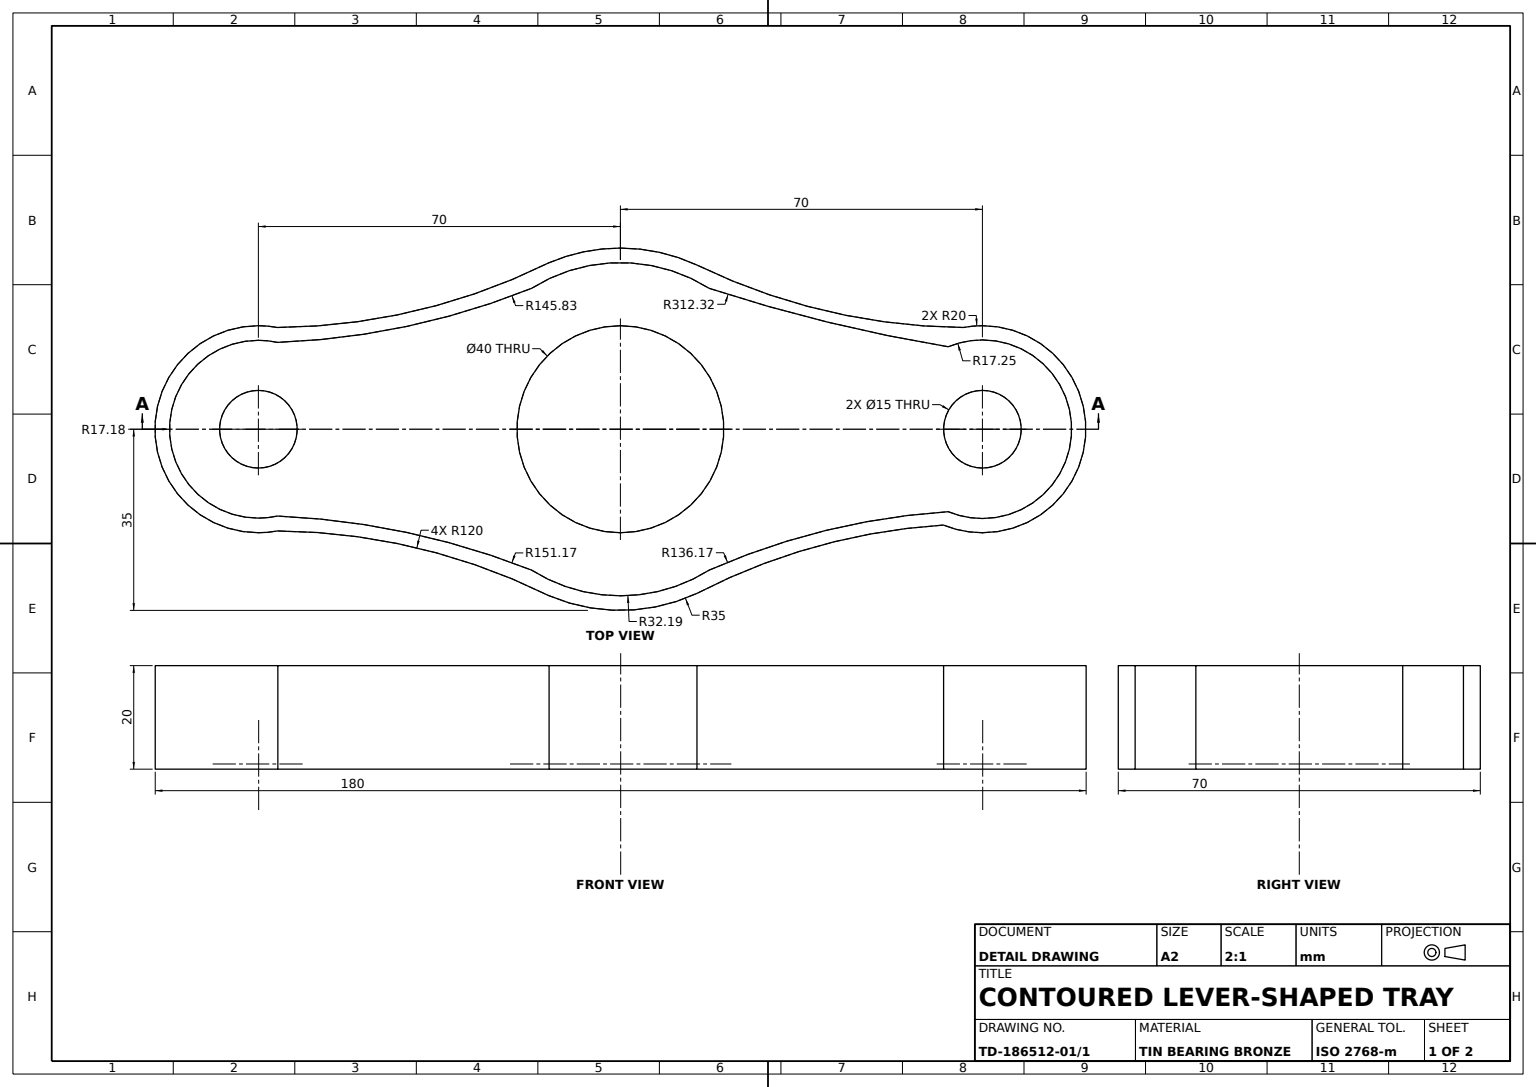
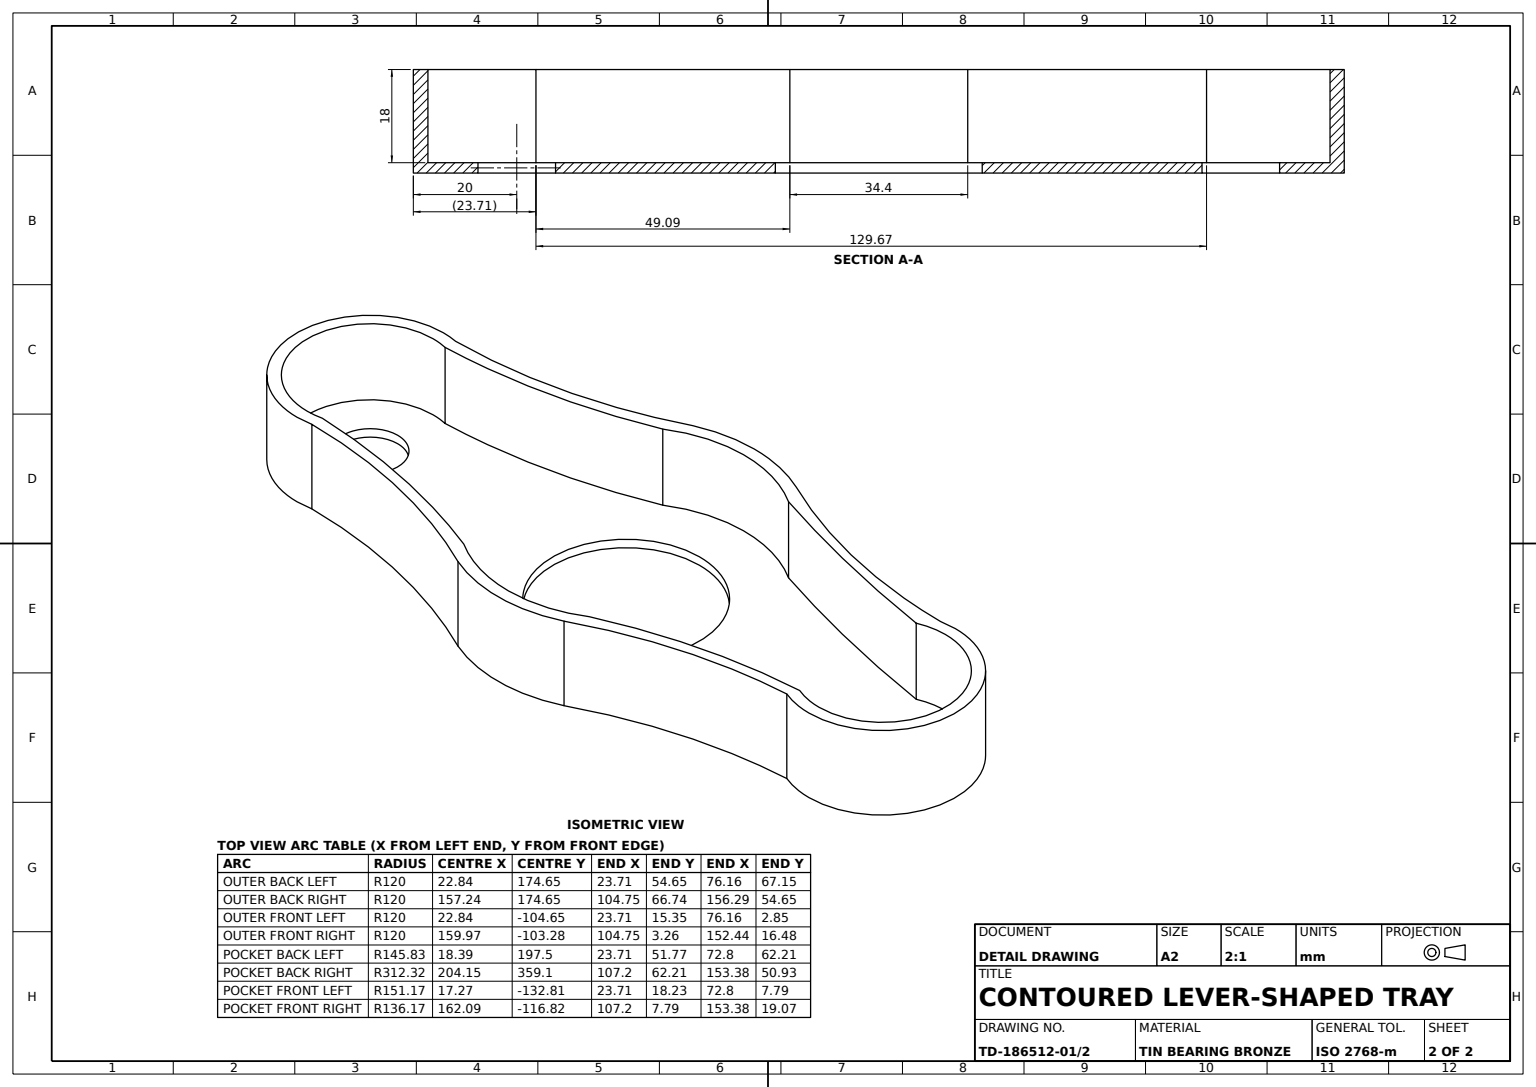
from build123d import *

# Parameters (mm, degrees)
PLATE_OUTLINE_AND_HOLES_SKETCH_R   = 7.5
PLATE_OUTLINE_AND_HOLES_SKETCH_R_2 = 20
PLATE_BODY_20MM_DEPTH              = 20
POCKET_18MM_DEEP_DEPTH             = 18


with BuildPart() as part:
    # Plate Outline and Holes Sketch → Plate Body 20mm (new body)
    with BuildSketch(Plane(origin=(0, 0, 0), x_dir=(1, 0, 0), z_dir=(0, 1, 0))):
        with BuildLine():
            ThreePointArc((0, -19.652996117), (25.514601751, -22.586747832), (49.820562895, -30.88265372))
            ThreePointArc((49.820562895, -30.88265372), (51.138080036, -31.506466617), (52.447922151, -32.146238124))
            ThreePointArc((52.447922151, -32.146238124), (66.786580153, -34.996485409), (81.03870417, -31.741030931))
            ThreePointArc((81.03870417, -31.741030931), (82.081542873, -31.206935864), (83.12954659, -30.683048174))
            ThreePointArc((83.12954659, -30.683048174), (105.326078872, -22.335617103), (128.730725009, -18.516168186))
            ThreePointArc((128.730725009, -18.516168186), (156.18959255, -2.007382475), (132.581174315, 19.652996117))
            ThreePointArc((132.581174315, 19.652996117), (106.605286262, 22.709869626), (81.908714055, 31.322102615))
            ThreePointArc((81.908714055, 31.322102615), (81.473287731, 31.530691668), (81.03870417, 31.741030931))
            ThreePointArc((81.03870417, 31.741030931), (66.786580153, 34.996485409), (52.447922151, 32.146238124))
            ThreePointArc((52.447922151, 32.146238124), (51.138080036, 31.506466617), (49.820562895, 30.88265372))
            ThreePointArc((49.820562895, 30.88265372), (25.514601751, 22.586747832), (0, 19.652996117))
            ThreePointArc((0, 19.652996117), (-23.709412843, 0), (0, -19.652996117))
        make_face()
        with Locations(Location((-3.709412843, 0, 0), (0, 0, 270))):
            Circle(PLATE_OUTLINE_AND_HOLES_SKETCH_R, mode=Mode.SUBTRACT)
        with Locations(Location((66.290587157, 0, 0), (0, 0, 270))):
            Circle(PLATE_OUTLINE_AND_HOLES_SKETCH_R_2, mode=Mode.SUBTRACT)
        with Locations(Location((136.290587157, 0, 0), (0, 0, 270))):
            Circle(PLATE_OUTLINE_AND_HOLES_SKETCH_R, mode=Mode.SUBTRACT)
    extrude(amount=PLATE_BODY_20MM_DEPTH)

    # Pocket Outline Sketch → Pocket 18mm Deep (cut)
    with BuildSketch(Plane(origin=(0, 20, 0), x_dir=(1, 0, 0), z_dir=(0, 1, 0))):
        with BuildLine():
            ThreePointArc((0, 16.772992409), (-20.887684525, 0), (0, -16.772992409))
            ThreePointArc((0, -16.772992409), (24.982456418, -19.938077439), (49.092914173, -27.206276583))
            ThreePointArc((49.092914173, -27.206276583), (66.290587157, -32.186044206), (83.488260142, -27.206276583))
            ThreePointArc((83.488260142, -27.206276583), (106.082407894, -19.537899767), (129.668226583, -15.931146045))
            ThreePointArc((129.668226583, -15.931146045), (153.543328212, 0), (129.668226583, 15.931146045))
            ThreePointArc((129.668226583, 15.931146045), (106.363417967, 20.688843047), (83.488260142, 27.206276583))
            ThreePointArc((83.488260142, 27.206276583), (66.290587157, 32.186044206), (49.092914173, 27.206276583))
            ThreePointArc((49.092914173, 27.206276583), (24.998686698, 19.861707266), (0, 16.772992409))
        make_face()
    extrude(amount=-POCKET_18MM_DEEP_DEPTH, mode=Mode.SUBTRACT)


solid = part.part
